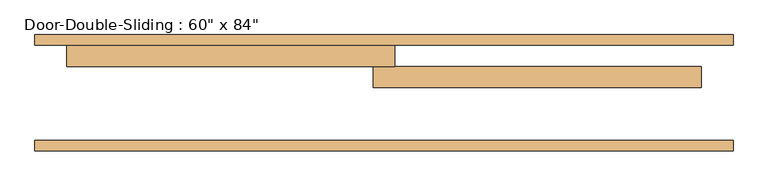
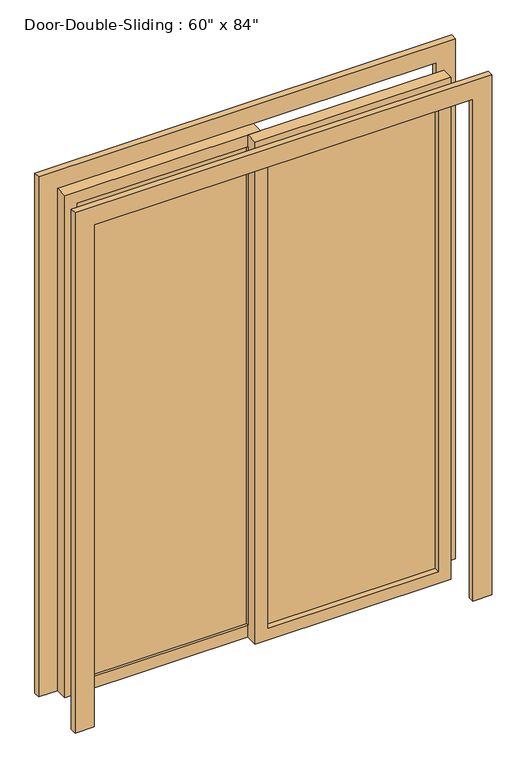
"""IFC4 building model written with IfcOpenShell, lengths in millimetres: door geometry."""

from ifc_helpers import new_model, si_unit, frame, origin, place, context, project, spatial, polyline, outline, extrude, source, transform, mapped, element, save


def door_238c678e(model_context):
    return source(origin(), model_context, "Body", "SweptSolid", [
        extrude(outline(polyline([(0.0, 838.2), (2209.8, 838.2), (2209.8, -838.2), (0.0, -838.2), (0.0, -762.0), (2133.6, -762.0), (2133.6, 762.0), (0.0, 762.0), (0.0, 838.2)])), frame((0.0, 241.3, 0.0), z_axis=(0.0, 1.0, 0.0), x_axis=(0.0, 0.0, 1.0)), (0.0, 0.0, 1.0), 25.4),
        extrude(outline(polyline([(0.0, -838.2), (0.0, -762.0), (2133.6, -762.0), (2133.6, 762.0), (0.0, 762.0), (0.0, 838.2), (2209.8, 838.2), (2209.8, -838.2), (0.0, -838.2)])), frame((0.0, -12.7, 0.0), z_axis=(0.0, 1.0, 0.0), x_axis=(0.0, 0.0, 1.0)), (0.0, 0.0, 1.0), 25.4),
        extrude(outline(polyline([(2133.6, 25.4), (2133.6, -762.0), (0.0, -762.0), (0.0, 25.4), (2133.6, 25.4)]), holes=[polyline([(2082.8, -25.4), (50.8, -25.4), (50.8, -711.2), (2082.8, -711.2), (2082.8, -25.4)])]), frame((0.0, 190.5, 0.0), z_axis=(0.0, 1.0, 0.0), x_axis=(0.0, 0.0, 1.0)), (0.0, 0.0, 1.0), 50.8),
        extrude(outline(polyline([(2133.6, -25.4), (0.0, -25.4), (0.0, 762.0), (2133.6, 762.0), (2133.6, -25.4)]), holes=[polyline([(2082.8, 25.4), (2082.8, 711.2), (50.8, 711.2), (50.8, 25.4), (2082.8, 25.4)])]), frame((0.0, 139.7, 0.0), z_axis=(0.0, 1.0, 0.0), x_axis=(0.0, 0.0, 1.0)), (0.0, 0.0, 1.0), 50.8),
        extrude(outline(polyline([(-25.4, 200.025), (-711.2, 200.025), (-711.2, 206.375), (-25.4, 206.375), (-25.4, 200.025)])), frame((0.0, 0.0, 50.8), z_axis=(0.0, 0.0, 1.0), x_axis=(1.0, 0.0, 0.0)), (0.0, 0.0, 1.0), 2032.0),
        extrude(outline(polyline([(25.4, 168.275), (711.2, 168.275), (711.2, 161.925), (25.4, 161.925), (25.4, 168.275)])), frame((0.0, 0.0, 50.8), z_axis=(0.0, 0.0, 1.0), x_axis=(1.0, 0.0, 0.0)), (0.0, 0.0, 1.0), 2032.0),
    ])


if __name__ == "__main__":
    model = new_model("IFC4")
    model_context = context("Model", 3, world=origin())
    ifc_project = project(units=[si_unit("LENGTHUNIT", "METRE", prefix="MILLI")], contexts=[model_context])
    site = spatial("IfcSite", under=ifc_project)
    building = spatial("IfcBuilding", under=site)
    placement = place(None, origin())
    door_shape = door_238c678e(model_context)
    element("IfcDoor", 1, ObjectType="Door-Double-Sliding : 60\" x 84\"", at=placement, inside=building, context=model_context, shape_type="MappedRepresentation", body=[
        mapped(door_shape, transform((0.0, 0.0, 0.0), x_axis=(1.0, 0.0, 0.0), y_axis=(0.0, 1.0, 0.0), z_axis=(0.0, 0.0, 1.0))),
    ])
    save(model, "model.ifc")

# Revit data of these elements
# Type "Door-Double-Sliding : 60\" x 84\""
#   Type Mark = "9"
#   Construction Type Id = "opn-d45"
#   Assembly Code = "C1020"
#   Analytic Construction = "Wood frame, double glass door "
#   Thickness = 0' - 2"
#   Thermal Resistance (R) = 1.8150 (h·ft²·°F)/BTU
#   Heat Transfer Coefficient (U) = 0.5510 BTU/(h·ft²·°F)
#   Height = 7' - 0"
#   Rail Width = 0' - 2"
#   Stiles = 0' - 2"
#   Trim Projection Ext = 0' - 1"
#   Trim Projection Int = 0' - 1"
#   Trim Width = 0' - 3"
#   Width = 5' - 0"
#   Define Thermal Properties by = 1
#   Glazing = Glass
#   Panel Material = Wood - Birch - Solid Stained Light Low Gloss
#   Trim Material = Paint - Sienna
#   Visual Light Transmittance = 0
#   Solar Heat Gain Coefficient = 0
#   Function = (empty or 0)
#   Wall Closure = (empty or 0)
# Element 1 (IfcDoor, "Door-Double-Sliding : 60\" x 84\"")
#   Materials on its faces: "Paint - Sienna", "Wood - Birch - Solid Stained Light Low Gloss", "Glass"
# Materials
#   "Glass": class "Glass", colour RGB 0 128 192, transparency 0.75, Description = "Soda Lime Glass", Cost = 0
#   "Wood - Birch - Solid Stained Light Low Gloss": class "Wood", colour RGB 210 159 95, transparency 0, Cost = 0
#   "Paint - Sienna": colour RGB 118 70 51, transparency 0, Cost = 0
